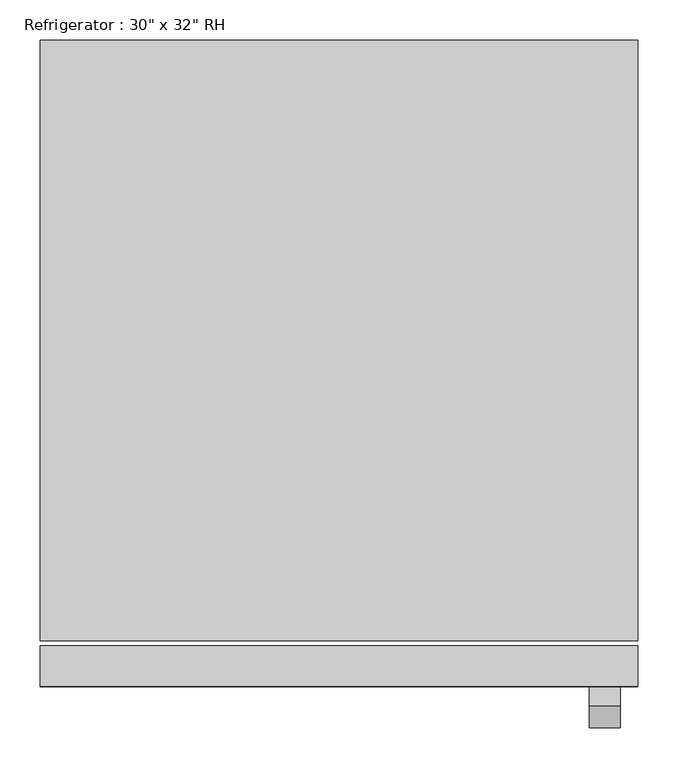
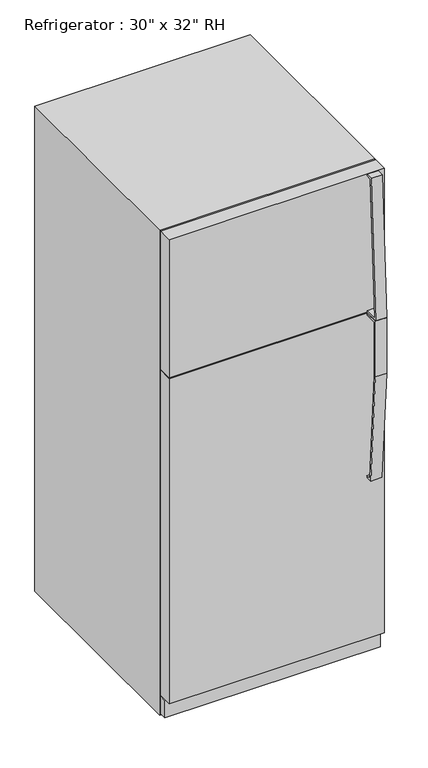
"""IFC4 building model written with IfcOpenShell, lengths in millimetres: proxy geometry."""

from ifc_helpers import new_model, si_unit, frame, origin, origin_with_axes, place, context, project, spatial, polyline, outline, extrude, source, transform, mapped, element, save


def proxy_a13a33b2(model_context):
    return source(origin(), model_context, "Body", "SweptSolid", [
        extrude(outline(polyline([(-417.9010285, 1262.0625), (-462.3510285, 1262.0625), (-462.3510285, 1065.4342469), (-434.8723987, 672.4715334), (-417.9010285, 672.4715334), (-417.9010285, 666.1370017), (-440.7949512, 666.1370017), (-468.7010285, 1065.2125), (-468.7010285, 1268.4125), (-417.9010285, 1268.4125), (-417.9010285, 1262.0625)])), frame((312.7375, 0.0, 0.0), z_axis=(1.0, 0.0, 0.0), x_axis=(0.0, 1.0, 0.0)), (0.0, 0.0, 1.0), 38.4332978),
        extrude(outline(polyline([(-442.739413, 1778.0), (-418.6780855, 1778.0), (-418.6780855, 1771.65), (-437.5263449, 1771.65), (-463.4007207, 1277.9375), (-418.6780855, 1277.9375), (-418.6780855, 1271.5875), (-469.2793675, 1271.5875), (-442.739413, 1778.0)])), frame((312.7375, 0.0, 0.0), z_axis=(1.0, 0.0, 0.0), x_axis=(0.0, 1.0, 0.0)), (0.0, 0.0, 1.0), 38.4332978),
        extrude(outline(polyline([(373.0625, -367.1010285), (373.0625, -392.5010285), (-373.0625, -392.5010285), (-373.0625, -367.1010285), (373.0625, -367.1010285)])), frame((0.0, 0.0, 9.3816357), z_axis=(0.0, 0.0, 1.0), x_axis=(1.0, 0.0, 0.0)), (0.0, 0.0, 1.0), 63.5),
        extrude(outline(polyline([(373.0625, -367.1010285), (373.0625, -417.9010285), (-373.0625, -417.9010285), (-373.0625, -367.1010285), (373.0625, -367.1010285)])), frame((0.0, 0.0, 76.2), z_axis=(0.0, 0.0, 1.0), x_axis=(1.0, 0.0, 0.0)), (0.0, 0.0, 1.0), 1192.2125),
        extrude(outline(polyline([(373.0625, -367.1010285), (373.0625, -417.9010285), (-373.0625, -417.9010285), (-373.0625, -367.1010285), (373.0625, -367.1010285)])), frame((0.0, 0.0, 1271.5875), z_axis=(0.0, 0.0, 1.0), x_axis=(1.0, 0.0, 0.0)), (0.0, 0.0, 1.0), 506.4125),
        extrude(outline(polyline([(373.0625, 388.5489715), (373.0625, -360.7510285), (-373.0625, -360.7510285), (-373.0625, 388.5489715), (373.0625, 388.5489715)])), origin_with_axes(), (0.0, 0.0, 1.0), 1778.0),
    ])


if __name__ == "__main__":
    model = new_model("IFC4")
    model_context = context("Model", 3, world=origin())
    ifc_project = project(units=[si_unit("LENGTHUNIT", "METRE", prefix="MILLI")], contexts=[model_context])
    site = spatial("IfcSite", under=ifc_project)
    building = spatial("IfcBuilding", under=site)
    placement = place(None, origin())
    proxy_shape = proxy_a13a33b2(model_context)
    element("IfcBuildingElementProxy", 1, Name="Refrigerator : 30\" x 32\" RH", ObjectType="Refrigerator : 30\" x 32\" RH", at=placement, inside=building, context=model_context, shape_type="MappedRepresentation", body=[
        mapped(proxy_shape, transform((0.0, 0.0, 0.0), x_axis=(1.0, 0.0, 0.0), y_axis=(0.0, 1.0, 0.0), z_axis=(0.0, 0.0, 1.0))),
    ])
    save(model, "model.ifc")

# Revit data of these elements
# Type "Refrigerator : 30\" x 32\" RH"
#   Label = "REF."
#   Assembly Code = "E1090400"
#   Depth = 2' - 7 3/4"
#   Handle = 2' - 3"
#   Height = 5' - 10"
#   Rear Clearance = 0' - 2"
#   Top Door Height = 1' - 8"
#   Width = 2' - 5 3/8"
#   Material = Carpet (1)
#   Default Elevation = 0
# Element 1 (IfcBuildingElementProxy, "Refrigerator : 30\" x 32\" RH")
#   Materials on its faces: "Carpet (1)", "Steel, Chrome Plated"
# Materials
#   "Carpet (1)": class "Carpet", colour RGB 124 80 67, transparency 0, Description = "Interior finish"
#   "Steel, Chrome Plated": class "Metal", colour RGB 17 17 17, transparency 0, Description = "Chromiuim plated steel", Cost = 0
